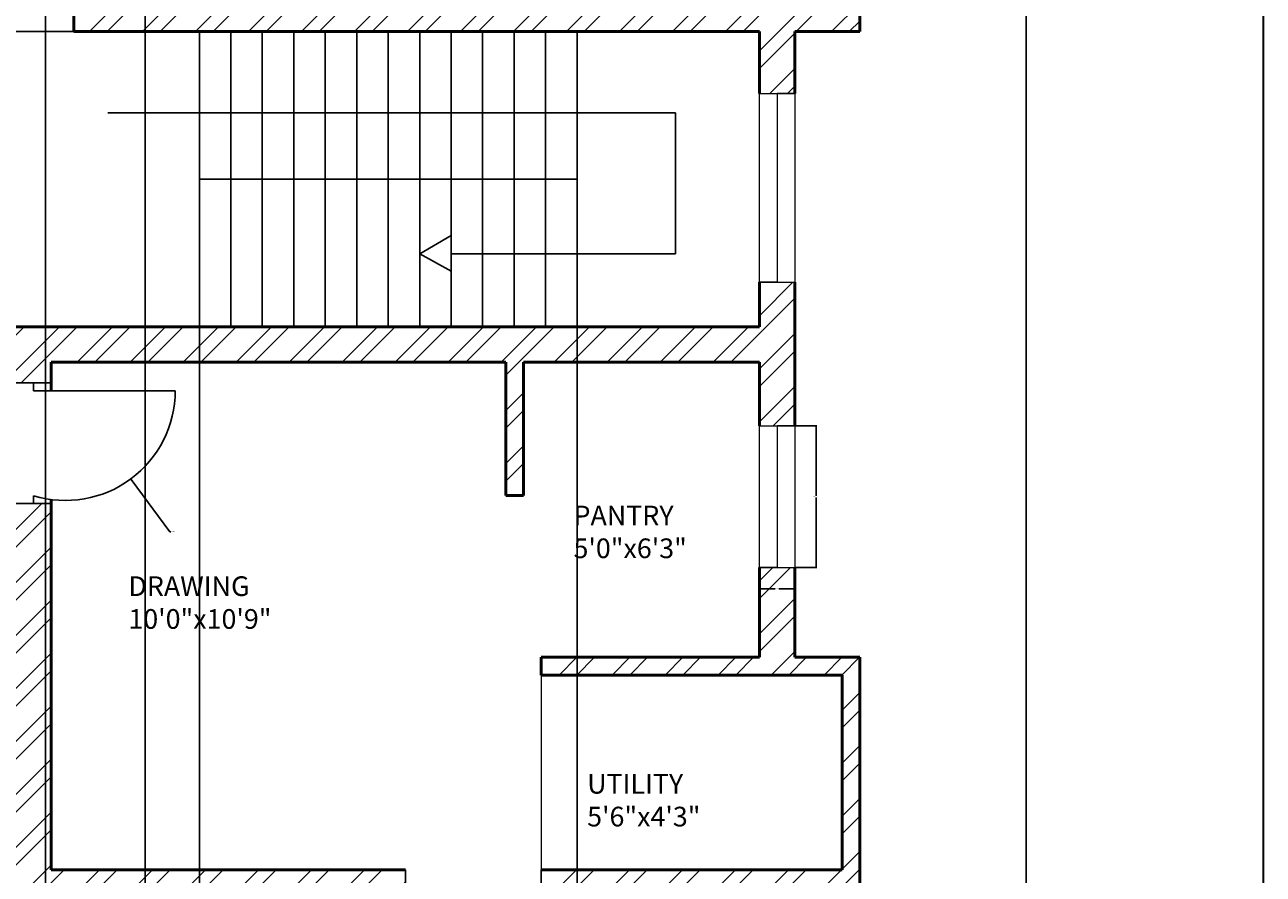
# Model space of a CAD drawing. Units: inches. Extents: x 1896 to 2572, y 1528 to 2474.
# Tile 5 of 10: x 2257 to 2572, y 1817 to 2033. Entities that reach past the tile are written whole.
import ezdxf

# ---------------------------------------------------------------- set-up
doc = ezdxf.new("R2010")
doc.units = ezdxf.units.IN
for name, color, linetype, lineweight in [('A-ANNO-DIMS', 2, 'Continuous', 18), ('A-ANNO-TTLB', 7, 'Continuous', 35), ('A-AREA-IDEN', 7, 'Continuous', 18), ('A-DOOR', 11, 'Continuous', 25), ('A-FLOR', 7, 'Continuous', 18), ('A-FLOR-STRS', 71, 'Continuous', 25), ('A-GLAZ', 131, 'Continuous', 20), ('A-WALL', 7, 'Continuous', 50)]:
    doc.layers.add(name, color=color, linetype=linetype, lineweight=lineweight)
doc.layers.add('A-WALL-PATT', color=215, linetype='Continuous', lineweight=13, true_color=0xa953a0)
doc.styles.get("Standard").update_dxf_attribs({"font": 'arial.ttf'})
doc.dimstyles.get("Standard").update_dxf_attribs({"dimtxt": 0.18, "dimasz": 0.18, "dimexe": 0.18, "dimexo": 0.0625, "dimgap": 0.09, "dimtad": 0, "dimtih": 1, "dimtoh": 1, "dimdec": 4, "dimzin": 0, "dimdsep": 46, "dimtxsty": 'Standard', "dimcen": 0.09, "dimadec": 0, "dimazin": 0, "dimtfac": 1, "dimtdec": 4, "dimtofl": 0, "dimtmove": 0, "dimatfit": 3, "dimfxl": 1, "dimtolj": 1, "dimtzin": 0, "dimarcsym": 0})

# ---------------------------------------------------------------- blocks, each defined once
blk = doc.blocks.new('WIN-36IN')
for p, q in [((0, 36), (9, 36)), ((0, 0), (0, 36)), ((9, 36), (4.5, 36)), ((4.5, 36), (4.5, 0)), ((9, 36), (9, 0)), ((4.5, 0), (0, 0)), ((0, 0), (9, 0))]:
    blk.add_line(p, q)
blk = doc.blocks.new('*D15')
at = {"layer": 'A-ANNO-DIMS', "color": 0, "lineweight": -2, "transparency": 16777216}
for p, q in [((2452.68, 1930.73), (2458.2, 1930.73)), ((2458.02, 1930.55), (2458.02, 1912.91)), ((2458.02, 1894.91), (2458.02, 1912.55)), ((2452.68, 1894.73), (2458.2, 1894.73))]:
    blk.add_line(p, q, dxfattribs=at)
at = {"layer": 'A-ANNO-DIMS', "color": 0, "transparency": 16777216}
for points in [[(2457.99, 1930.55), (2458.05, 1930.55), (2458.02, 1930.73)], [(2457.99, 1894.91), (2458.05, 1894.91), (2458.02, 1894.73)]]:
    blk.add_solid(points, dxfattribs=at)
at = {"layer": 'Defpoints', "color": 0, "transparency": 16777216}
for p in [(2452.62, 1930.73), (2458.02, 1930.73), (2452.62, 1894.73)]:
    blk.add_point(p, dxfattribs=at)
at = {"layer": 'A-ANNO-DIMS', "color": 0, "transparency": 16777216, "insert": (2458.02, 1912.73), "char_height": 0.18, "attachment_point": 5}
blk.add_mtext('\\A1;WDW 36 TYP.', dxfattribs=at)
blk = doc.blocks.new('*D16')
at = {"layer": 'A-ANNO-DIMS', "color": 0, "lineweight": -2, "transparency": 16777216}
for p, q in [((2443.62, 1894.67), (2443.62, 1889.15)), ((2452.62, 1894.67), (2452.62, 1889.15)), ((2443.8, 1889.33), (2447.66, 1889.33)), ((2452.44, 1889.33), (2448.58, 1889.33))]:
    blk.add_line(p, q, dxfattribs=at)
at = {"layer": 'A-ANNO-DIMS', "color": 0, "transparency": 16777216}
for points in [[(2443.8, 1889.36), (2443.8, 1889.3), (2443.62, 1889.33)], [(2452.44, 1889.36), (2452.44, 1889.3), (2452.62, 1889.33)]]:
    blk.add_solid(points, dxfattribs=at)
at = {"layer": 'Defpoints', "color": 0, "transparency": 16777216}
for p in [(2443.62, 1894.73), (2452.62, 1894.73), (2452.62, 1889.33)]:
    blk.add_point(p, dxfattribs=at)
at = {"layer": 'A-ANNO-DIMS', "color": 0, "transparency": 16777216, "insert": (2448.12, 1889.33), "char_height": 0.18, "attachment_point": 5}
blk.add_mtext('\\A1;9 TYP.', dxfattribs=at)
blk = doc.blocks.new('*D20')
at = {"layer": 'A-ANNO-DIMS', "color": 0, "lineweight": -2, "transparency": 16777216}
for p, q in [((2180.68, 2431.4), (2511.65, 2431.4)), ((2511.47, 2431.22), (2511.47, 2049.83)), ((2511.47, 1668.08), (2511.47, 2049.47)), ((2452.68, 1667.9), (2511.65, 1667.9))]:
    blk.add_line(p, q, dxfattribs=at)
at = {"layer": 'A-ANNO-DIMS', "color": 0, "transparency": 16777216}
for points in [[(2511.44, 2431.22), (2511.5, 2431.22), (2511.47, 2431.4)], [(2511.44, 1668.08), (2511.5, 1668.08), (2511.47, 1667.9)]]:
    blk.add_solid(points, dxfattribs=at)
at = {"layer": 'Defpoints', "color": 0, "transparency": 16777216}
for p in [(2180.62, 2431.4), (2511.47, 2431.4), (2452.62, 1667.9)]:
    blk.add_point(p, dxfattribs=at)
at = {"layer": 'A-ANNO-DIMS', "color": 0, "transparency": 16777216, "insert": (2511.47, 2049.65), "char_height": 0.18, "attachment_point": 5}
blk.add_mtext('\\A1;763.5', dxfattribs=at)
blk = doc.blocks.new('*D31')
at = {"layer": 'A-ANNO-DIMS', "color": 0, "lineweight": -2, "transparency": 16777216}
for p, q in [((2301.2, 2030.9), (1919.59, 2030.9)), ((1919.77, 2030.72), (1919.77, 1993.58)), ((1919.77, 1956.08), (1919.77, 1993.22)), ((2301.2, 1955.9), (1919.59, 1955.9))]:
    blk.add_line(p, q, dxfattribs=at)
at = {"layer": 'A-ANNO-DIMS', "color": 0, "transparency": 16777216}
for points in [[(1919.74, 2030.72), (1919.8, 2030.72), (1919.77, 2030.9)], [(1919.74, 1956.08), (1919.8, 1956.08), (1919.77, 1955.9)]]:
    blk.add_solid(points, dxfattribs=at)
at = {"layer": 'Defpoints', "color": 0, "transparency": 16777216}
for p in [(1919.77, 2030.9), (2301.26, 2030.9), (2301.26, 1955.9)]:
    blk.add_point(p, dxfattribs=at)
at = {"layer": 'A-ANNO-DIMS', "color": 0, "transparency": 16777216, "insert": (1919.77, 1993.4), "char_height": 0.18, "attachment_point": 5}
blk.add_mtext('\\A1;75', dxfattribs=at)
blk = doc.blocks.new('*D32')
at = {"layer": 'A-ANNO-DIMS', "color": 0, "lineweight": -2, "transparency": 16777216}
for p, q in [((2301.26, 1955.84), (2301.26, 1549.1)), ((2397.26, 1955.84), (2397.26, 1549.1)), ((2301.44, 1549.28), (2349.04, 1549.28)), ((2397.08, 1549.28), (2349.48, 1549.28))]:
    blk.add_line(p, q, dxfattribs=at)
at = {"layer": 'A-ANNO-DIMS', "color": 0, "transparency": 16777216}
for points in [[(2301.44, 1549.31), (2301.44, 1549.25), (2301.26, 1549.28)], [(2397.08, 1549.31), (2397.08, 1549.25), (2397.26, 1549.28)]]:
    blk.add_solid(points, dxfattribs=at)
at = {"layer": 'Defpoints', "color": 0, "transparency": 16777216}
for p in [(2301.26, 1955.9), (2397.26, 1955.9), (2397.26, 1549.28)]:
    blk.add_point(p, dxfattribs=at)
at = {"layer": 'A-ANNO-DIMS', "color": 0, "transparency": 16777216, "insert": (2349.26, 1549.28), "char_height": 0.18, "attachment_point": 5}
blk.add_mtext('\\A1;96', dxfattribs=at)
blk = doc.blocks.new('*D35')
at = {"layer": 'A-ANNO-DIMS', "color": 0, "lineweight": -2, "transparency": 16777216}
for p, q in [((2262.12, 2373.34), (2262.12, 1549.1)), ((2287.46, 2373.34), (2287.46, 1549.1)), ((2262.3, 1549.28), (2274.4, 1549.28)), ((2287.28, 1549.28), (2275.19, 1549.28))]:
    blk.add_line(p, q, dxfattribs=at)
at = {"layer": 'A-ANNO-DIMS', "color": 0, "transparency": 16777216}
for points in [[(2262.3, 1549.31), (2262.3, 1549.25), (2262.12, 1549.28)], [(2287.28, 1549.31), (2287.28, 1549.25), (2287.46, 1549.28)]]:
    blk.add_solid(points, dxfattribs=at)
at = {"layer": 'Defpoints', "color": 0, "transparency": 16777216}
for p in [(2262.12, 2373.4), (2287.46, 2373.4), (2287.46, 1549.28)]:
    blk.add_point(p, dxfattribs=at)
at = {"layer": 'A-ANNO-DIMS', "color": 0, "transparency": 16777216, "insert": (2274.79, 1549.28), "char_height": 0.18, "attachment_point": 5}
blk.add_mtext('\\A1;25.34', dxfattribs=at)
blk = doc.blocks.new('*D40')
at = {"layer": 'A-ANNO-DIMS', "color": 0, "lineweight": -2, "transparency": 16777216}
for p, q in [((2267.16, 1939.64), (2267.34, 1939.64)), ((2267.25, 1939.55), (2267.25, 1939.73)), ((2293.79, 1903.8), (2283.95, 1917.09)), ((2293.97, 1903.8), (2293.79, 1903.8))]:
    blk.add_line(p, q, dxfattribs=at)
at = {"layer": 'A-ANNO-DIMS', "color": 0, "transparency": 16777216}
blk.add_solid([(2283.97, 1917.11), (2283.92, 1917.07), (2283.84, 1917.24)], dxfattribs=at)
at = {"layer": 'Defpoints', "color": 0, "transparency": 16777216}
for p in [(2267.25, 1939.64), (2283.84, 1917.24)]:
    blk.add_point(p, dxfattribs=at)
at = {"layer": 'A-ANNO-DIMS', "color": 0, "transparency": 16777216, "insert": (2294.52, 1903.8), "char_height": 0.18, "attachment_point": 5}
blk.add_mtext('\\A1;R27.873', dxfattribs=at)

msp = doc.modelspace()

# ---------------------------------------------------------------- hatches: boundary and pattern name
at = {"layer": 'A-WALL-PATT'}
h = msp.add_hatch(dxfattribs=at)
h.set_pattern_fill('ANSI32', color=256)
h.paths.add_polyline_path([(2071.6224, 2382.3979), (2071.6224, 2422.3979), (2110.6224, 2422.3979), (2110.6224, 2382.3979), (2110.6224, 2357.5961), (2119.6224, 2357.5961), (2119.6224, 2422.3979), (2171.6224, 2422.3979), (2171.6224, 2373.3979), (2193.5093, 2373.3979), (2193.5093, 2377.8979), (2193.5093, 2382.3979), (2180.6224, 2382.3979), (2180.6224, 2431.3979), (2171.6224, 2431.3979), (2119.6224, 2431.3979), (2110.6224, 2431.3979), (2062.6224, 2431.3979), (2062.6224, 2422.3979), (2062.6224, 2382.3979), (1978.6224, 2382.3979), (1978.6224, 2313.0337), (1987.6224, 2313.0337), (1987.6224, 2373.3979), (2062.6224, 2373.3979), (2067.1224, 2373.3979), (2067.1224, 2353.7982), (2071.6224, 2353.8883)])
h.paths.add_polyline_path([(2287.4624, 2382.3979), (2229.5093, 2382.3979), (2229.5093, 2373.3979), (2253.1224, 2373.3979), (2253.1224, 2175.8979), (2247.1039, 2175.8979), (2247.1039, 2166.8979), (2253.1224, 2166.8979), (2253.1224, 2150.8283), (2262.1224, 2150.8283), (2262.1224, 2166.8979), (2262.1224, 2236.8979), (2349.0731, 2236.8979), (2349.0731, 2239.1479), (2349.0731, 2241.3979), (2262.1224, 2241.3979), (2262.1224, 2373.3979), (2287.4624, 2373.3979)])
h.paths.add_polyline_path([(2452.6224, 2382.3979), (2347.4624, 2382.3979), (2347.4624, 2373.3979), (2382.1224, 2373.3979), (2382.1224, 2334.0335), (2386.6224, 2334.0335), (2386.6224, 2373.3979), (2443.6224, 2373.3979), (2443.6224, 2316.2056), (2452.6224, 2316.2056)])
h.paths.add_polyline_path([(2452.6224, 2292.2056), (2448.1224, 2292.2056), (2443.6224, 2292.2056), (2443.6224, 2292.0047), (2443.6224, 2280.9372), (2443.6224, 2268.3979), (2386.6224, 2268.3979), (2386.6224, 2312.4044), (2384.3724, 2312.4044), (2382.1224, 2312.4044), (2382.1224, 2241.3979), (2379.1336, 2241.3979), (2379.1336, 2236.8979), (2386.6224, 2236.8979), (2386.6224, 2263.8979), (2443.6224, 2263.8979), (2443.6224, 2248.8449), (2452.6224, 2248.8449)])
h.paths.add_polyline_path([(2364.1285, 2116.8979), (2262.1224, 2116.8979), (2262.1224, 2120.5401), (2257.6224, 2120.5401), (2253.1224, 2120.5401), (2253.1224, 2107.8979), (2262.1224, 2107.8979), (2269.354, 2107.8979), (2269.354, 2094.0702), (2278.354, 2094.0702), (2278.354, 2107.8979), (2347.6224, 2107.8979), (2347.6224, 2039.8979), (2278.354, 2039.8979), (2278.354, 2054.7605), (2269.354, 2054.7605), (2269.354, 2030.8979), (2278.354, 2030.8979), (2443.6224, 2030.8979), (2443.6224, 2015.198), (2452.6224, 2015.198), (2452.6224, 2030.8979), (2464.6224, 2030.8979), (2469.1224, 2030.8979), (2469.1224, 2117.0352), (2452.6767, 2116.9466), (2452.6285, 2125.8979), (2452.6224, 2125.8979), (2452.6224, 2212.8449), (2443.6224, 2212.8449), (2443.6224, 2116.8979), (2385.832, 2116.8979), (2385.832, 2112.3979), (2385.832, 2107.8979), (2464.6224, 2107.8979), (2464.6224, 2039.8979), (2443.6224, 2039.8979), (2356.6224, 2039.8979), (2356.6224, 2107.8979), (2364.1285, 2107.8979)])
h.paths.add_polyline_path([(2452.6224, 1967.198), (2443.6224, 1967.198), (2443.6224, 1955.8979), (2259.1224, 1955.8979), (2254.6224, 1955.8979), (2254.6224, 1941.6358), (2263.6224, 1941.6358), (2263.6224, 1946.8979), (2379.1224, 1946.8979), (2379.1224, 1913.0204), (2383.6224, 1913.0204), (2383.6224, 1946.8979), (2443.6224, 1946.8979), (2443.6224, 1930.729), (2452.6224, 1930.729)])
h.paths.add_polyline_path([(2469.1224, 1871.8979), (2464.6224, 1871.8979), (2452.6224, 1871.8979), (2452.6224, 1894.729), (2443.6224, 1894.729), (2443.6224, 1871.8979), (2388.1304, 1871.8979), (2388.1304, 1867.3979), (2443.6224, 1867.3979), (2464.6224, 1867.3979), (2464.6224, 1817.8979), (2443.6224, 1817.8979), (2388.1304, 1817.8979), (2388.1304, 1815.6479), (2388.1304, 1813.3979), (2391.1224, 1813.3979), (2391.1224, 1747.8899), (2395.6224, 1747.8899), (2395.6224, 1813.3979), (2443.6224, 1813.3979), (2443.6224, 1781.4434), (2452.6224, 1781.4434), (2452.6224, 1813.3979), (2464.6224, 1813.3979), (2469.1224, 1813.3979)])
h.paths.add_polyline_path([(2263.6224, 1910.9737), (2259.1224, 1910.9737), (2254.6224, 1910.9737), (2254.6224, 1889.8979), (2251.2778, 1889.8979), (2251.2778, 1880.8979), (2254.6224, 1880.8979), (2254.6224, 1817.8979), (2254.6224, 1754.8979), (2254.6224, 1693.3979), (2254.6224, 1684.3979), (2254.6224, 1672.3979), (2200.6224, 1672.3979), (2200.6224, 1684.3979), (2200.6224, 1693.3979), (2200.6224, 1754.8979), (2196.1224, 1754.8979), (2196.1224, 1693.3979), (2150.0488, 1693.3979), (2150.0488, 1684.3979), (2196.1224, 1684.3979), (2196.1224, 1672.3979), (2196.1224, 1667.8979), (2254.6224, 1667.8979), (2259.1224, 1667.8979), (2259.1224, 1693.3979), (2259.1224, 1813.3979), (2353.6224, 1813.3979), (2353.6224, 1815.6479), (2353.6224, 1817.8979), (2263.6224, 1817.8979)])
h.paths.add_polyline_path([(2391.1224, 1693.3979), (2345.6981, 1693.3979), (2345.6981, 1684.3979), (2391.1224, 1684.3979)])
h.paths.add_polyline_path([(2285.6981, 1693.3979), (2259.1224, 1693.3979), (2259.1224, 1684.3979), (2285.6981, 1684.3979), (2285.6981, 1688.8979)], flags=17)
h.paths.add_polyline_path([(2452.6224, 1757.4434), (2448.1224, 1757.4434), (2443.6224, 1757.4434), (2443.6224, 1726.3979), (2395.6224, 1726.3979), (2395.6224, 1728.6572), (2393.3724, 1728.6572), (2391.1224, 1728.6572), (2391.1224, 1717.6723), (2395.6224, 1717.6723), (2395.6224, 1721.8979), (2443.6224, 1721.8979), (2443.6224, 1714.8), (2452.6224, 1714.8)])
h.paths.add_polyline_path([(2452.6224, 1684.3979), (2452.6224, 1690.8), (2443.6224, 1690.8), (2443.6224, 1679.8979), (2443.6224, 1672.3979), (2395.6224, 1672.3979), (2395.6224, 1695.6708), (2391.1224, 1695.5986), (2391.1224, 1672.3979), (2391.1224, 1667.8979), (2452.6224, 1667.8979)])
h.paths.add_polyline_path([(1987.6224, 1880.8979), (2068.6224, 1880.8979), (2125.6224, 1880.8979), (2125.6224, 1788.8466), (2130.1224, 1788.8466), (2130.1224, 1880.8979), (2216.1958, 1880.8979), (2216.1958, 1885.3979), (2216.1958, 1889.8979), (2208.1224, 1889.8979), (2208.1224, 1996.3717), (2203.6224, 1996.3717), (2199.1224, 1996.3717), (2199.1224, 1889.8979), (2073.1224, 1889.8979), (2073.1224, 1917.1874), (2068.6224, 1917.1874), (2068.6224, 1889.8979), (1987.6224, 1889.8979), (1987.6224, 1912.4976), (1978.6224, 1912.4976), (1978.6224, 1805.5193), (1987.6224, 1805.5193)])
h.paths.add_polyline_path([(2019.9303, 1754.8979), (1987.6224, 1754.8979), (1966.6224, 1754.8979), (1966.6224, 1801.0193), (1987.6224, 1801.0193), (1987.6224, 1805.5193), (1962.1224, 1805.5193), (1962.1224, 1750.3979), (1966.6224, 1750.3979), (1978.6224, 1750.3979), (1987.6224, 1750.3979), (2019.9303, 1750.3979)])
h.paths.add_polyline_path([(2135.5566, 1754.8979), (2130.1224, 1754.8979), (2130.1224, 1758.052), (2127.8724, 1758.052), (2125.6224, 1758.052), (2125.6224, 1754.8979), (2068.6224, 1754.8979), (2043.2292, 1754.8979), (2043.2292, 1750.3979), (2068.6224, 1750.3979), (2098.6224, 1750.3979), (2098.6224, 1693.3979), (2068.6224, 1693.3979), (1987.6224, 1693.3979), (1987.6224, 1707.3003), (1983.1224, 1707.3003), (1978.6224, 1707.3003), (1978.6224, 1684.3979), (2068.6224, 1684.3979), (2126.0488, 1684.3979), (2126.0488, 1688.8979), (2126.0488, 1693.3979), (2103.1224, 1693.3979), (2103.1224, 1750.3979), (2130.1224, 1750.3979), (2135.5566, 1750.3979)])
h.paths.add_polyline_path([(1987.6224, 1750.3979), (1978.6224, 1750.3979), (1978.6224, 1731.3003), (1987.6224, 1731.3003)], flags=0)
h.paths.add_polyline_path([(1987.6224, 1973.8979), (2068.6224, 1973.8979), (2073.1224, 1973.8979), (2073.1224, 1978.3979), (1971.1224, 1978.3979), (1971.1224, 2030.3979), (1978.6224, 2030.3979), (1987.6224, 2030.3979), (2104.9199, 2030.3979), (2104.9199, 2032.6479), (2104.9199, 2034.8979), (1987.6224, 2034.8979), (1971.1224, 2034.8979), (1971.1224, 2085.8979), (2003.6464, 2085.8979), (2003.6464, 2090.3979), (1987.6224, 2090.3979), (1987.6224, 2166.8979), (2115.1224, 2166.8979), (2137.6224, 2166.8979), (2137.6224, 2114.4229), (2142.1224, 2114.4229), (2142.1224, 2124.8979), (2153.5306, 2124.8979), (2153.5306, 2127.1479), (2153.5306, 2129.3979), (2142.1224, 2129.3979), (2142.1224, 2166.8979), (2199.1224, 2166.8979), (2199.1224, 2129.3979), (2177.5306, 2129.3979), (2177.5306, 2124.8979), (2199.1224, 2124.8979), (2199.1224, 2034.8979), (2142.1224, 2034.8979), (2142.1224, 2091.6671), (2139.8724, 2091.6671), (2137.6224, 2091.6671), (2137.6224, 2034.8979), (2133.8326, 2034.8979), (2133.8326, 2030.3979), (2137.6224, 2030.3979), (2142.1224, 2030.3979), (2199.1224, 2030.3979), (2199.1224, 2024.2654), (2208.1224, 2024.2654), (2208.1224, 2030.3979), (2208.1224, 2166.8979), (2214.5775, 2166.8979), (2214.5775, 2171.3979), (2214.5775, 2175.8979), (2115.1224, 2175.8979), (2115.1224, 2329.9154), (2112.4137, 2329.9154), (2110.6224, 2329.9154), (2110.6224, 2175.8979), (2082.1224, 2175.8979), (2082.1224, 2202.6443), (2079.8724, 2202.6443), (2077.6224, 2202.6443), (2077.6224, 2175.8979), (1987.6224, 2175.8979), (1987.6224, 2191.3531), (1983.1224, 2191.3531), (1978.6224, 2191.3531), (1978.6224, 2090.3979), (1966.6224, 2090.3979), (1966.6224, 2085.8979), (1966.6224, 2030.3979), (1966.6224, 1973.8979), (1978.6224, 1973.8979), (1978.6224, 1948.4976), (1983.1224, 1948.4976), (1987.6224, 1948.4976)])
h.paths.add_polyline_path([(1987.6224, 2253.0337), (1983.1224, 2253.0337), (1978.6224, 2253.0337), (1978.6224, 2215.3531), (1987.6224, 2215.3531), (1987.6224, 2224.8979), (2077.6224, 2224.8979), (2077.6224, 2221.9854), (2082.1224, 2221.9854), (2082.1224, 2229.3979), (1987.6224, 2229.3979)], flags=17)
h.paths.add_polyline_path([(2220.5047, 1978.7278), (2253.7278, 1978.7278), (2253.7278, 1997.3851), (2220.5047, 1997.3851)], flags=9)
h.paths.add_polyline_path([(2303.6746, 2064.9806), (2320.5334, 2064.9806), (2320.5334, 2075.2842), (2303.6746, 2075.2842)], flags=25)

# ---------------------------------------------------------------- linework, layer by layer
at = {"layer": 'A-ANNO-TTLB'}
msp.add_lwpolyline([(1895.84, 2455.9668), (2571.702, 2455.9668), (2571.702, 1527.8833), (1895.84, 1527.8833)], close=True, dxfattribs=at)
at = {"layer": 'A-DOOR'}
for p, q in [((2254.6224, 1941.6358), (2263.6224, 1941.6358)), ((2263.6224, 1941.6358), (2259.1224, 1941.6358)), ((2259.1224, 1941.6358), (2259.1224, 1939.6358)), ((2259.1224, 1939.6358), (2295.1224, 1939.6358)), ((2259.1224, 1910.9737), (2259.1224, 1912.9737)), ((2254.6224, 1910.9737), (2263.6224, 1910.9737)), ((2263.6224, 1910.9737), (2259.1224, 1910.9737)), ((2353.6224, 1817.8979), (2353.6224, 1813.3979)), ((2388.1304, 1813.3979), (2388.1304, 1817.8979)), ((2388.1304, 1817.8979), (2388.1304, 1815.6479))]:
    msp.add_line(p, q, dxfattribs=at)
msp.add_arc((2267.2492, 1939.6358), 27.8732, 253.048462, 0, dxfattribs=at)
at = {"layer": 'A-FLOR'}
msp.add_line((2388.1304, 1869.6479), (2388.1304, 1817.8979), dxfattribs=at)
at = {"layer": 'A-FLOR-STRS'}
for p, q in [((2301.2636, 2030.8979), (2301.2636, 1955.8979)), ((2309.2636, 2030.8979), (2309.2636, 1955.8979)), ((2317.2636, 2030.8979), (2317.2636, 1955.8979)), ((2325.2636, 2030.8979), (2325.2636, 1955.8979)), ((2333.2636, 2030.8979), (2333.2636, 1955.8979)), ((2341.2636, 2030.8979), (2341.2636, 1955.8979)), ((2349.2636, 2030.8979), (2349.2636, 1955.8979)), ((2357.2636, 2030.8979), (2357.2636, 1955.8979)), ((2365.2636, 2030.8979), (2365.2636, 1955.8979)), ((2373.2636, 2030.8979), (2373.2636, 1955.8979)), ((2381.2636, 2030.8979), (2381.2636, 1955.8979)), ((2389.2636, 2030.8979), (2389.2636, 1955.8979)), ((2397.2636, 2030.8979), (2397.2636, 1955.8979)), ((2278.0272, 2010.2811), (2422.2644, 2010.2811)), ((2422.2644, 2010.2811), (2422.2644, 1974.4284)), ((2397.2636, 1993.3979), (2301.2636, 1993.3979)), ((2397.2636, 1955.8979), (2397.2636, 1993.3979)), ((2357.2636, 1974.4284), (2365.2636, 1979.0586)), ((2365.2636, 1979.0586), (2365.2636, 1970.0111)), ((2365.2636, 1970.0111), (2357.2636, 1974.4284)), ((2422.2644, 1974.4284), (2365.2636, 1974.4284))]:
    msp.add_line(p, q, dxfattribs=at)
at = {"layer": 'A-GLAZ'}
for p, q in [((2443.6224, 2015.198), (2452.6224, 2015.198)), ((2443.6224, 1967.198), (2443.6224, 2015.198)), ((2452.6224, 2015.198), (2448.1224, 2015.198)), ((2448.1224, 2015.198), (2448.1224, 1967.198)), ((2452.6224, 2015.198), (2452.6224, 1967.198)), ((2448.1224, 1967.198), (2443.6224, 1967.198)), ((2443.6224, 1967.198), (2452.6224, 1967.198))]:
    msp.add_line(p, q, dxfattribs=at)
at = {"layer": 'A-WALL'}
for p, q in [((2469.1224, 2030.8979), (2469.1224, 2116.8979)), ((2269.354, 2030.8979), (2269.354, 2054.7605)), ((2269.354, 2030.8979), (2443.6224, 2030.8979)), ((2278.354, 2030.8979), (2269.354, 2030.8979)), ((2443.6224, 2030.8979), (2443.6224, 2015.198)), ((2452.6224, 2030.8979), (2464.6224, 2030.8979)), ((2452.6224, 2030.8979), (2452.6224, 2015.198)), ((2464.6224, 2030.8979), (2469.1224, 2030.8979)), ((2443.6224, 1967.198), (2443.6224, 1955.8979)), ((2452.6224, 1967.198), (2452.6224, 1930.729)), ((2254.6224, 1955.8979), (2263.6224, 1955.8979)), ((2443.6224, 1955.8979), (2259.1224, 1955.8979)), ((2263.6224, 1946.8979), (2263.6224, 1939.6358)), ((2379.1224, 1946.8979), (2263.6224, 1946.8979)), ((2379.1224, 1913.0204), (2379.1224, 1946.8979)), ((2443.6224, 1946.8979), (2383.6224, 1946.8979)), ((2443.6224, 1946.8979), (2383.6224, 1946.8979)), ((2383.6224, 1946.8979), (2383.6224, 1913.0204)), ((2443.6224, 1946.8979), (2443.6224, 1930.729)), ((2263.6224, 1911.9996), (2263.6224, 1817.8979)), ((2379.1224, 1913.0204), (2383.6224, 1913.0204)), ((2443.6224, 1894.729), (2443.6224, 1871.8979)), ((2452.6224, 1894.729), (2452.6224, 1871.8979)), ((2388.1304, 1871.8979), (2443.6224, 1871.8979)), ((2388.1304, 1867.3979), (2388.1304, 1871.8979)), ((2452.6224, 1871.8979), (2464.6224, 1871.8979)), ((2469.1224, 1871.8979), (2464.6224, 1871.8979)), ((2469.1224, 1813.3979), (2469.1224, 1871.8979)), ((2443.6224, 1867.3979), (2388.1304, 1867.3979)), ((2443.6224, 1867.3979), (2464.6224, 1867.3979)), ((2464.6224, 1867.3979), (2464.6224, 1817.8979)), ((2353.6224, 1817.8979), (2263.6224, 1817.8979)), ((2443.6224, 1817.8979), (2388.1304, 1817.8979)), ((2464.6224, 1817.8979), (2443.6224, 1817.8979))]:
    msp.add_line(p, q, dxfattribs=at)

# ---------------------------------------------------------------- block references
at = {"layer": 'A-GLAZ'}
msp.add_blockref('WIN-36IN', (2443.622, 1894.729), dxfattribs=at)

# ---------------------------------------------------------------- texts
at = {"layer": 'A-AREA-IDEN', "char_height": 5, "attachment_point": 1}
for s, width, insert in [('PANTRY\\P5\'0"x6\'3"', 79.756703, (2396.3724, 1910.4361)), ('DRAWING\\P10\'0"x10\'9"', 160.404515, (2283.2179, 1892.4767)), ('UTILITY\\P5\'6"x4\'3"', 119.352616, (2399.8382, 1842.2531))]:
    msp.add_mtext_dynamic_manual_height_columns(s, width=width, gutter_width=12.5, heights=[0], dxfattribs=dict(at, insert=insert))

# ---------------------------------------------------------------- dimensions: what is measured, and where the dimension line sits
at = {"layer": 'A-ANNO-DIMS'}
for base, p1, p2, override, picture, middle in [((2511.4724, 2431.3979), (2452.6224, 1667.8979), (2180.6224, 2431.3979), {"dimdec": 1, "dimlfac": 1, "dimrnd": 0, "dimzin": 0, "dimdsep": 46, "dimlunit": 2}, '*D20', (2511.4724, 2049.6479)), ((1919.7724, 2030.8979), (2301.2636, 1955.8979), (2301.2636, 2030.8979), {"dimdec": 0, "dimlfac": 1, "dimrnd": 0, "dimzin": 0, "dimdsep": 46, "dimlunit": 2}, '*D31', (1919.7724, 1993.3979))]:
    dim = msp.add_linear_dim(base=base, p1=p1, p2=p2, angle=90, dimstyle='Standard', override=override, dxfattribs=at)
    dim.commit()
    dim.dimension.update_dxf_attribs({"geometry": picture, "text_midpoint": middle})
for base, p1, p2, override, picture, middle in [((2287.4624, 1549.2803), (2262.1224, 2373.3979), (2287.4624, 2373.3979), {"dimdec": 2, "dimlfac": 1, "dimrnd": 0, "dimzin": 0, "dimdsep": 46, "dimlunit": 2}, '*D35', (2274.7924, 1549.2803)), ((2397.2636, 1549.2803), (2301.2636, 1955.8979), (2397.2636, 1955.8979), {"dimdec": 0, "dimlfac": 1, "dimrnd": 0, "dimzin": 0, "dimdsep": 46, "dimlunit": 2}, '*D32', (2349.2636, 1549.2803))]:
    dim = msp.add_linear_dim(base=base, p1=p1, p2=p2, dimstyle='Standard', override=override, dxfattribs=at)
    dim.commit()
    dim.dimension.update_dxf_attribs({"geometry": picture, "text_midpoint": middle})
dim = msp.add_radius_dim(center=(2267.2492, 1939.6358), mpoint=(2283.8382, 1917.2367), dimstyle='Standard', override={"dimdec": 3, "dimlfac": 1, "dimrnd": 0, "dimzin": 0, "dimdsep": 46, "dimlunit": 2}, dxfattribs=at)
dim.commit()
dim.dimension.update_dxf_attribs({"geometry": '*D40', "text_midpoint": (2294.5214, 1903.7972), "dimtype": 164})
dim = msp.add_linear_dim(base=(2458.0224, 1930.729), p1=(2452.6224, 1894.729), p2=(2452.6224, 1930.729), angle=90, text='WDW <> TYP.', dimstyle='Standard', override={"dimdec": 0, "dimlfac": 1, "dimrnd": 0, "dimzin": 0, "dimdsep": 46, "dimlunit": 2}, dxfattribs=at)
dim.commit()
dim.dimension.update_dxf_attribs({"geometry": '*D15', "text_midpoint": (2458.0224, 1912.729)})
dim = msp.add_linear_dim(base=(2452.6224, 1889.329), p1=(2443.6224, 1894.729), p2=(2452.6224, 1894.729), text='<> TYP.', dimstyle='Standard', override={"dimdec": 0, "dimlfac": 1, "dimrnd": 0, "dimzin": 0, "dimdsep": 46, "dimlunit": 2}, dxfattribs=at)
dim.commit()
dim.dimension.update_dxf_attribs({"geometry": '*D16', "text_midpoint": (2448.1224, 1889.329)})

doc.saveas('drawing.dxf')
